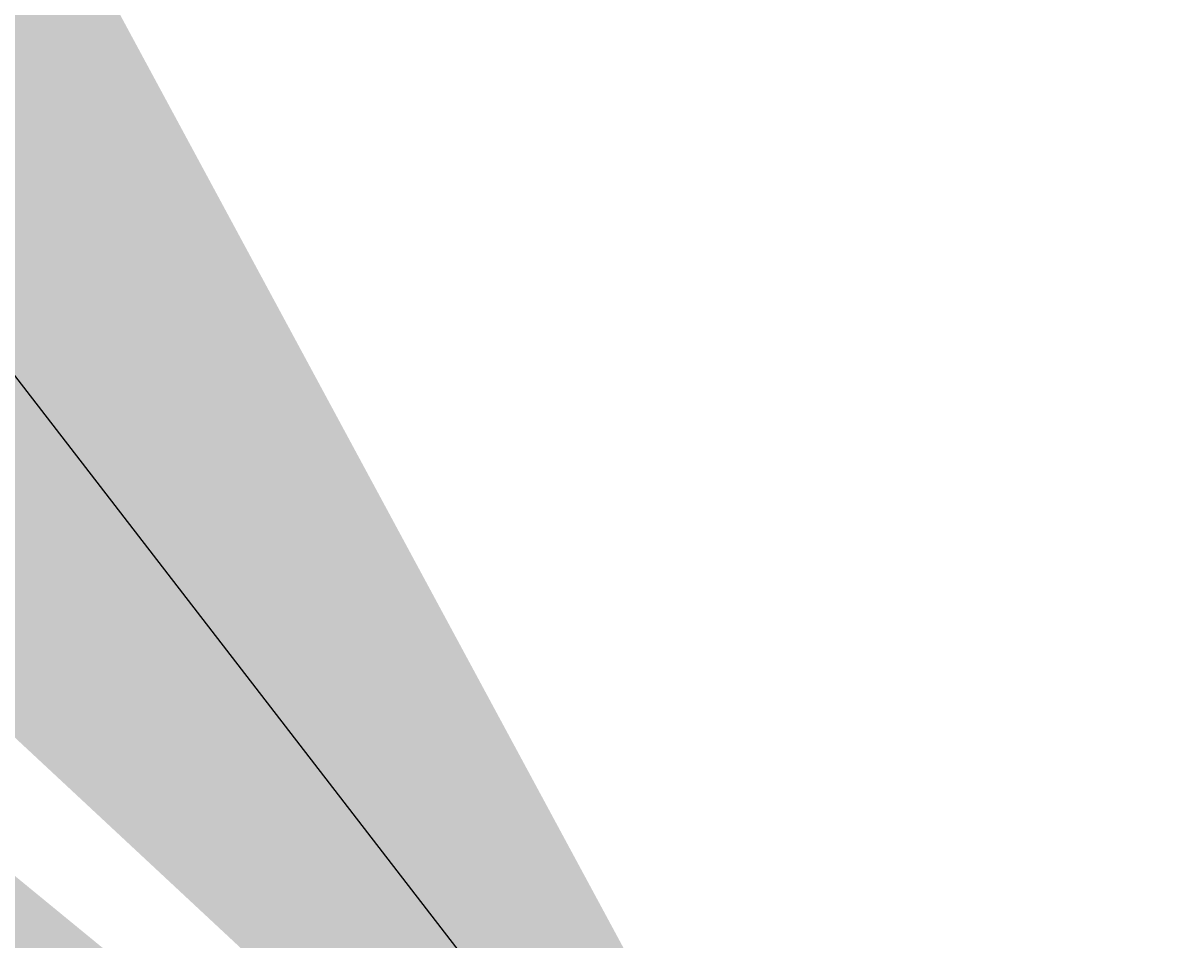
# Model space of a CAD drawing. Units: inches. Extents: x -9413 to 9703, y -9719 to 9096.
# Tile 1 of 1: x -2479 to 493, y 2041 to 4393. Entities that reach past the tile are written whole.
import ezdxf
from ezdxf import colors
from ezdxf.entities.mleader import LeaderData, LeaderLine
from ezdxf.math import Vec2, Vec3

# ---------------------------------------------------------------- set-up
doc = ezdxf.new("R2010")
doc.units = ezdxf.units.IN
doc.header["$MEASUREMENT"] = 0
doc.layers.add('M-ANNO-TEXT', color=7, linetype='Continuous', lineweight=18)
doc.styles.get("Standard").update_dxf_attribs({"font": 'arial.ttf'})

msp = doc.modelspace()

# ---------------------------------------------------------------- leaders
at = {"layer": 'M-ANNO-TEXT'}
ml = msp.add_multileader_mtext('Standard', dxfattribs=at)
ml.set_content('steam drum', color=256)
ml.set_leader_properties()
ml.build(insert=Vec2(0, 0))
ml.multileader.update_dxf_attribs({"dogleg_length": 0.36, "arrow_head_size": 10000, "scale": 10})
ctx = ml.context
ctx.base_point, ctx.scale, ctx.char_height, ctx.arrow_head_size, ctx.landing_gap_size, ctx.plane_origin = Vec3(1.078100315116472, 187.1657656808087), 10, 5.4, 10000, 0.9, Vec3(56.53630785249729, 178.1917761520126)
ctx.text_align_type = 2
notes = []
notes.append((ctx, [(0, (1, 1, 0), (49.60206616053652, 187.1657656808087), (-1, 0), 7.616326009130828, [(0, [(56.5363078524973, 178.1917761520126)], 0, [])])]))
ctx.mtext.insert, ctx.mtext.alignment, ctx.mtext.flow_direction = Vec3(41.08574015140569, 189.9099675907678), 3, 5
ml = msp.add_multileader_mtext('Standard', dxfattribs=at)
ml.set_content('Reheater', color=256)
ml.set_leader_properties()
ml.build(insert=Vec2(0, 0))
ml.multileader.update_dxf_attribs({"dogleg_length": 0.36, "arrow_head_size": 10000, "scale": 10})
ctx = ml.context
ctx.base_point, ctx.scale, ctx.char_height, ctx.arrow_head_size, ctx.landing_gap_size, ctx.plane_origin = Vec3(234.1414050860131, 159.7303554673012), 10, 5.4, 10000, 0.9, Vec3(221.1444910066821, 154.3050445940477)
notes.append((ctx, [(0, (1, 1, 0), (230.5414050860131, 159.7303554673012), (1, 0), 3.599999999999999, [(0, [(221.1444910066821, 154.3050445940477)], 0, [])])]))
ctx.mtext.insert, ctx.mtext.flow_direction = Vec3(235.0414050860131, 162.4745573772603), 5
ml = msp.add_multileader_mtext('Standard', dxfattribs=at)
ml.set_content('Boiler', color=256)
ml.set_leader_properties()
ml.build(insert=Vec2(0, 0))
ml.multileader.update_dxf_attribs({"dogleg_length": 0.36, "arrow_head_size": 10000, "scale": 10})
ctx = ml.context
ctx.base_point, ctx.scale, ctx.char_height, ctx.arrow_head_size, ctx.landing_gap_size, ctx.plane_origin = Vec3(31.04430257849453, 103.0991380116177), 10, 5.4, 10000, 0.9, Vec3(69.11352005531556, 99.3051261342938)
ctx.text_align_type = 2
notes.append((ctx, [(0, (1, 1, 0), (62.54209871927075, 103.0991380116177), (-1, 0), 10.86041551321825, [(0, [(69.11352005531556, 99.3051261342938)], 0, [])])]))
ctx.mtext.insert, ctx.mtext.alignment, ctx.mtext.flow_direction = Vec3(50.7816832060525, 105.8433399215768), 3, 5
for ctx, leaders in notes:
    for number, flags, end, landing, length, lines in leaders:
        leader = LeaderData()
        leader.index, (leader.has_last_leader_line, leader.has_dogleg_vector, leader.attachment_direction) = number, flags
        leader.last_leader_point, leader.dogleg_vector, leader.dogleg_length = Vec3(end), Vec3(landing), length
        for number, points, colour, breaks in lines:
            line = LeaderLine()
            line.index, line.vertices, line.color, line.breaks = number, Vec3.list(points), colors.encode_raw_color(colour), breaks
            leader.lines.append(line)
        ctx.leaders.append(leader)

doc.saveas('drawing.dxf')
